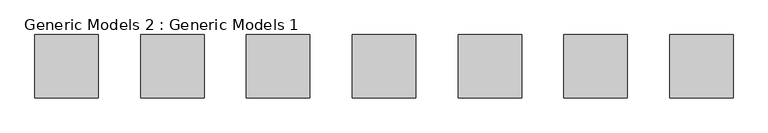
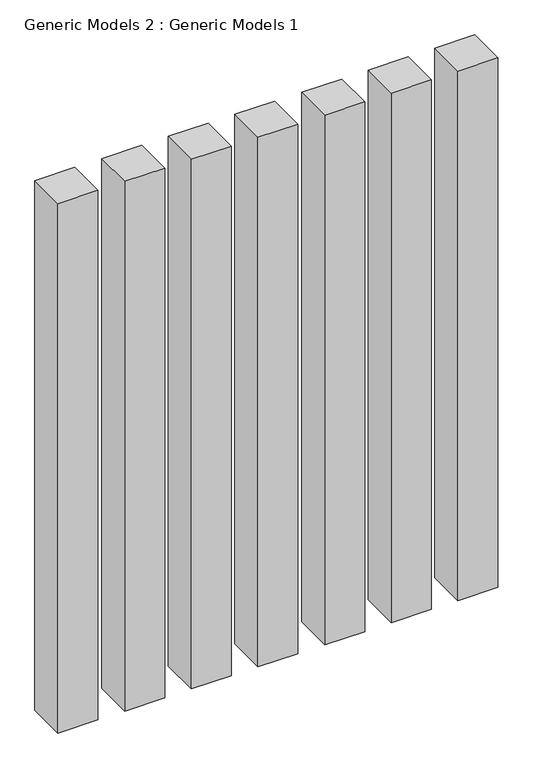
"""IFC4 building model written with IfcOpenShell, lengths in millimetres: proxy geometry, Generic Models 2 : Generic Models 1."""

from ifc_helpers import new_model, si_unit, origin, origin_with_axes, place, context, project, spatial, polyline, outline, extrude, source, transform, mapped, element, save


def generic_models_2_generic_models_1_d649346d(model_context):
    return source(origin(), model_context, "Body", "SweptSolid", [
        extrude(outline(polyline([(27378.0546318, -2836.165108), (27149.4546318, -2836.165108), (27149.4546318, -2607.565108), (27378.0546318, -2607.565108), (27378.0546318, -2836.165108)])), origin_with_axes(), (0.0, 0.0, 1.0), 3200.4),
        extrude(outline(polyline([(27759.0546318, -2836.165108), (27530.4546318, -2836.165108), (27530.4546318, -2607.565108), (27759.0546318, -2607.565108), (27759.0546318, -2836.165108)])), origin_with_axes(), (0.0, 0.0, 1.0), 3200.4),
        extrude(outline(polyline([(28140.0546318, -2836.165108), (27911.4546318, -2836.165108), (27911.4546318, -2607.565108), (28140.0546318, -2607.565108), (28140.0546318, -2836.165108)])), origin_with_axes(), (0.0, 0.0, 1.0), 3200.4),
        extrude(outline(polyline([(28521.0546318, -2836.165108), (28292.4546318, -2836.165108), (28292.4546318, -2607.565108), (28521.0546318, -2607.565108), (28521.0546318, -2836.165108)])), origin_with_axes(), (0.0, 0.0, 1.0), 3200.4),
        extrude(outline(polyline([(28902.0546318, -2836.165108), (28673.4546318, -2836.165108), (28673.4546318, -2607.565108), (28902.0546318, -2607.565108), (28902.0546318, -2836.165108)])), origin_with_axes(), (0.0, 0.0, 1.0), 3200.4),
        extrude(outline(polyline([(29283.0546318, -2836.165108), (29054.4546318, -2836.165108), (29054.4546318, -2607.565108), (29283.0546318, -2607.565108), (29283.0546318, -2836.165108)])), origin_with_axes(), (0.0, 0.0, 1.0), 3200.4),
        extrude(outline(polyline([(29664.0546318, -2836.165108), (29435.4546318, -2836.165108), (29435.4546318, -2607.565108), (29664.0546318, -2607.565108), (29664.0546318, -2836.165108)])), origin_with_axes(), (0.0, 0.0, 1.0), 3200.4),
    ])


if __name__ == "__main__":
    model = new_model("IFC4")
    model_context = context("Model", 3, world=origin())
    ifc_project = project(units=[si_unit("LENGTHUNIT", "METRE", prefix="MILLI")], contexts=[model_context])
    site = spatial("IfcSite", under=ifc_project)
    building = spatial("IfcBuilding", under=site)
    placement = place(None, origin())
    generic_models_2_generic_models_1_shape = generic_models_2_generic_models_1_d649346d(model_context)
    element("IfcBuildingElementProxy", 1, Name="Generic Models 2 : Generic Models 1", ObjectType="Generic Models 2 : Generic Models 1", at=placement, inside=building, context=model_context, shape_type="MappedRepresentation", body=[
        mapped(generic_models_2_generic_models_1_shape, transform((0.0, 0.0, 0.0), x_axis=(1.0, 0.0, 0.0), y_axis=(0.0, 1.0, 0.0), z_axis=(0.0, 0.0, 1.0))),
    ])
    save(model, "model.ifc")

# Revit data of these elements
# Element 1 (IfcBuildingElementProxy, "Generic Models 2 : Generic Models 1")
#   Materials on its faces: "0 olive green"
# Materials
#   "0 olive green": class "Generic", colour RGB 120 120 120, transparency 0, Cost = 0
